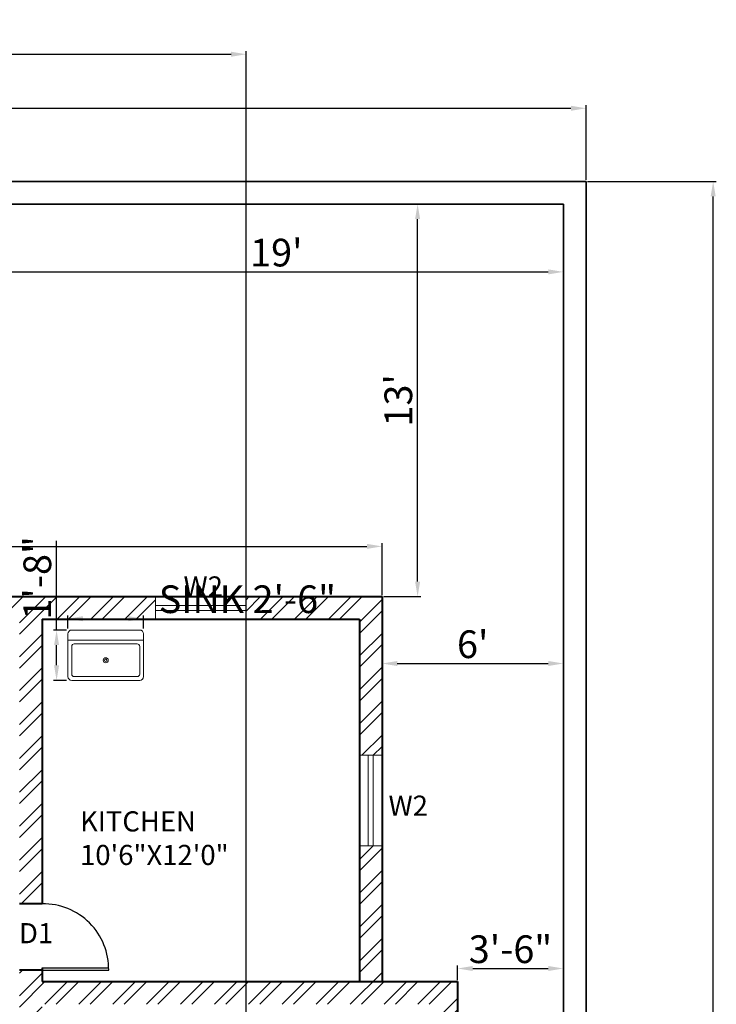
# Model space of a CAD drawing. Units: inches. Extents: x 2069 to 3028, y 691 to 1726.
# Tile 10 of 10: x 2622 to 2899, y 1325 to 1717. Entities that reach past the tile are written whole.
import ezdxf

# ---------------------------------------------------------------- set-up
doc = ezdxf.new("R2010")
doc.units = ezdxf.units.IN
for name, color, linetype, lineweight in [('A-ANNO-DIMS', 2, 'Continuous', 18), ('A-DOOR', 3, 'Continuous', 25), ('A-FLOR-FIXT', 9, 'Continuous', 20), ('A-GLAZ', 4, 'Continuous', 20), ('A-WALL', 7, 'Continuous', 40), ('L-SITE-WALL', 7, 'Continuous', 35)]:
    doc.layers.add(name, color=color, linetype=linetype, lineweight=lineweight)
for name, color, linetype, lineweight, true_color in [('A-ANNO-TEXT', 11, 'Continuous', 18, 0xf27172), ('A-AREA-IDEN', 11, 'Continuous', 25, 0xf27172), ('A-WALL-PATT', 143, 'Continuous', 13, 0x7aafdf)]:
    doc.layers.add(name, color=color, linetype=linetype, lineweight=lineweight, true_color=true_color)
doc.styles.get("Standard").update_dxf_attribs({"font": 'arial.ttf'})
doc.dimstyles.new('ISO-25', dxfattribs={"dimtxt": 11, "dimasz": 6, "dimexe": 1.25, "dimexo": 0.625, "dimtad": 1, "dimlunit": 3, "dimtxsty": 'Standard', "dimcen": 2.5, "dimclrd": 3, "dimclre": 5, "dimclrt": 6, "dimadec": 0, "dimazin": 0, "dimtfac": 1, "dimtmove": 0, "dimatfit": 3, "dimfxl": 1, "dimarcsym": 0})

# ---------------------------------------------------------------- blocks, each defined once
blk = doc.blocks.new('Sink-single - 30 in top')
blk.add_line((-15, -3.999996), (15, -3.999996))
for points in [[(-13.5, 0), (13.5, 0)], [(-15, -18.499996), (-15, -1.5)], [(15, -1.5), (15, -18.499996)], [(-13.5, -17.499996), (-13.5, -6.499996)], [(-12.5, -5.499996), (12.5, -5.499996)], [(13.5, -6.499996), (13.5, -17.499996)], [(12.5, -18.499996), (-12.5, -18.499996)], [(13.5, -19.999996), (-13.5, -19.999996)]]:
    blk.add_lwpolyline(points)
for radius in [1, 0.5]:
    blk.add_circle((0, -11.999996), radius)
for centre, radius, start, end in [((-13.5, -1.5), 1.5, 90, 180), ((13.5, -1.5), 1.5, 0, 90), ((-12.5, -6.499996), 1, 90, 180), ((12.5, -6.499996), 1, 0, 90), ((-13.5, -18.499996), 1.5, 180, 270), ((-12.5, -17.499996), 1, 180, 270), ((12.5, -17.499996), 1, 270, 0), ((13.5, -18.499996), 1.5, 270, 0)]:
    blk.add_arc(centre, radius, start, end)
blk = doc.blocks.new('*D20')
at = {"layer": 'A-ANNO-DIMS', "color": 0, "lineweight": -2, "transparency": 16777216}
for p, q in [((2141.95, 1653.01), (2141.95, 1682.68)), ((2846.95, 1653.01), (2846.95, 1682.68)), ((2147.95, 1681.43), (2840.95, 1681.43))]:
    blk.add_line(p, q, dxfattribs=at)
at = {"layer": 'A-ANNO-DIMS', "color": 0, "transparency": 16777216}
for points in [[(2147.95, 1682.43), (2147.95, 1680.43), (2141.95, 1681.43)], [(2840.95, 1682.43), (2840.95, 1680.43), (2846.95, 1681.43)]]:
    blk.add_solid(points, dxfattribs=at)
at = {"layer": 'Defpoints', "color": 0, "transparency": 16777216}
for p in [(2846.95, 1681.43), (2141.95, 1652.39), (2846.95, 1652.39)]:
    blk.add_point(p, dxfattribs=at)
at = {"layer": 'A-ANNO-DIMS', "color": 0, "transparency": 16777216, "insert": (2494.45, 1687.67), "char_height": 11, "attachment_point": 5}
blk.add_mtext('58\'-9"', dxfattribs=at)
blk = doc.blocks.new('*D21')
at = {"layer": 'A-ANNO-DIMS', "color": 0, "lineweight": -2, "transparency": 16777216}
for p, q in [((2766.58, 1643.39), (2781.31, 1643.39)), ((2780.06, 1493.39), (2780.06, 1637.39)), ((2766.58, 1487.39), (2781.31, 1487.39))]:
    blk.add_line(p, q, dxfattribs=at)
at = {"layer": 'A-ANNO-DIMS', "color": 0, "transparency": 16777216}
for points in [[(2779.06, 1637.39), (2781.06, 1637.39), (2780.06, 1643.39)], [(2779.06, 1493.39), (2781.06, 1493.39), (2780.06, 1487.39)]]:
    blk.add_solid(points, dxfattribs=at)
at = {"layer": 'Defpoints', "color": 0, "transparency": 16777216}
for p in [(2765.95, 1643.39), (2780.06, 1643.39), (2765.95, 1487.39)]:
    blk.add_point(p, dxfattribs=at)
at = {"layer": 'A-ANNO-DIMS', "color": 0, "transparency": 16777216, "insert": (2773.82, 1565.39), "char_height": 11, "attachment_point": 5, "rotation": 90}
blk.add_mtext("13'", dxfattribs=at)
blk = doc.blocks.new('*D22')
at = {"layer": 'A-ANNO-DIMS', "color": 0, "lineweight": -2, "transparency": 16777216}
for p, q in [((2609.95, 1642.76), (2609.95, 1615.16)), ((2837.95, 1642.76), (2837.95, 1615.16)), ((2615.95, 1616.41), (2831.95, 1616.41))]:
    blk.add_line(p, q, dxfattribs=at)
at = {"layer": 'A-ANNO-DIMS', "color": 0, "transparency": 16777216}
for points in [[(2615.95, 1617.41), (2615.95, 1615.41), (2609.95, 1616.41)], [(2831.95, 1617.41), (2831.95, 1615.41), (2837.95, 1616.41)]]:
    blk.add_solid(points, dxfattribs=at)
at = {"layer": 'Defpoints', "color": 0, "transparency": 16777216}
for p in [(2609.95, 1643.39), (2837.95, 1643.39), (2837.95, 1616.41)]:
    blk.add_point(p, dxfattribs=at)
at = {"layer": 'A-ANNO-DIMS', "color": 0, "transparency": 16777216, "insert": (2723.95, 1622.65), "char_height": 11, "attachment_point": 5}
blk.add_mtext("19'", dxfattribs=at)
blk = doc.blocks.new('*D23')
at = {"layer": 'A-ANNO-DIMS', "color": 0, "lineweight": -2, "transparency": 16777216}
for p, q in [((2297.95, 1488.01), (2297.95, 1508.59)), ((2303.95, 1507.34), (2759.95, 1507.34)), ((2765.95, 1488.01), (2765.95, 1508.59))]:
    blk.add_line(p, q, dxfattribs=at)
at = {"layer": 'A-ANNO-DIMS', "color": 0, "transparency": 16777216}
for points in [[(2303.95, 1508.34), (2303.95, 1506.34), (2297.95, 1507.34)], [(2759.95, 1508.34), (2759.95, 1506.34), (2765.95, 1507.34)]]:
    blk.add_solid(points, dxfattribs=at)
at = {"layer": 'Defpoints', "color": 0, "transparency": 16777216}
for p in [(2765.95, 1507.34), (2297.95, 1487.39), (2765.95, 1487.39)]:
    blk.add_point(p, dxfattribs=at)
at = {"layer": 'A-ANNO-DIMS', "color": 0, "transparency": 16777216, "insert": (2531.95, 1513.58), "char_height": 11, "attachment_point": 5}
blk.add_mtext("39'", dxfattribs=at)
blk = doc.blocks.new('*D24')
at = {"layer": 'A-ANNO-DIMS', "color": 0, "lineweight": -2, "transparency": 16777216}
for p, q in [((2795.95, 1335.01), (2795.95, 1340.86)), ((2801.95, 1339.61), (2831.95, 1339.61)), ((2837.95, 1335.01), (2837.95, 1340.86))]:
    blk.add_line(p, q, dxfattribs=at)
at = {"layer": 'A-ANNO-DIMS', "color": 0, "transparency": 16777216}
for points in [[(2801.95, 1340.61), (2801.95, 1338.61), (2795.95, 1339.61)], [(2831.95, 1340.61), (2831.95, 1338.61), (2837.95, 1339.61)]]:
    blk.add_solid(points, dxfattribs=at)
at = {"layer": 'Defpoints', "color": 0, "transparency": 16777216}
for p in [(2837.95, 1339.61), (2795.95, 1334.39), (2837.95, 1334.39)]:
    blk.add_point(p, dxfattribs=at)
at = {"layer": 'A-ANNO-DIMS', "color": 0, "transparency": 16777216, "insert": (2816.95, 1345.85), "char_height": 11, "attachment_point": 5}
blk.add_mtext('3\'-6"', dxfattribs=at)
blk = doc.blocks.new('*D25')
at = {"layer": 'A-ANNO-DIMS', "color": 0, "lineweight": -2, "transparency": 16777216}
for p, q in [((2765.95, 1486.76), (2765.95, 1459.55)), ((2837.95, 1486.76), (2837.95, 1459.55)), ((2771.95, 1460.8), (2831.95, 1460.8))]:
    blk.add_line(p, q, dxfattribs=at)
at = {"layer": 'A-ANNO-DIMS', "color": 0, "transparency": 16777216}
for points in [[(2771.95, 1461.8), (2771.95, 1459.8), (2765.95, 1460.8)], [(2831.95, 1461.8), (2831.95, 1459.8), (2837.95, 1460.8)]]:
    blk.add_solid(points, dxfattribs=at)
at = {"layer": 'Defpoints', "color": 0, "transparency": 16777216}
for p in [(2765.95, 1487.39), (2837.95, 1487.39), (2837.95, 1460.8)]:
    blk.add_point(p, dxfattribs=at)
at = {"layer": 'A-ANNO-DIMS', "color": 0, "transparency": 16777216, "insert": (2801.95, 1467.04), "char_height": 11, "attachment_point": 5}
blk.add_mtext("6'", dxfattribs=at)
blk = doc.blocks.new('DOOR-SWING-26_4IN')
for p, q in [((0, 0), (-26.4, 0)), ((0, -1), (-26.4, -1))]:
    blk.add_line(p, q)
blk.add_arc((-0.5, -0.5), 25.9, 178.894, 271.106)
blk = doc.blocks.new('WINDOW-36IN')
for p, q in [((0, 0), (9, 0)), ((3.5, 0), (3.5, -36)), ((5.5, 0), (5.5, -36)), ((0, -36), (9, -36))]:
    blk.add_line(p, q)
blk = doc.blocks.new('*D74')
at = {"layer": 'A-ANNO-DIMS', "color": 5, "lineweight": -2, "transparency": 16777216}
for p, q in [((2641.15, 1474.73), (2641.15, 1479.86)), ((2671.15, 1474.73), (2671.15, 1479.86))]:
    blk.add_line(p, q, dxfattribs=at)
at = {"layer": 'A-ANNO-DIMS', "color": 3, "lineweight": -2, "transparency": 16777216}
for p, q in [((2647.15, 1478.61), (2665.15, 1478.61)), ((2671.15, 1478.61), (2747.73, 1478.61))]:
    blk.add_line(p, q, dxfattribs=at)
at = {"layer": 'A-ANNO-DIMS', "color": 3, "transparency": 16777216}
for points in [[(2647.15, 1479.61), (2647.15, 1477.61), (2641.15, 1478.61)], [(2665.15, 1479.61), (2665.15, 1477.61), (2671.15, 1478.61)]]:
    blk.add_solid(points, dxfattribs=at)
at = {"layer": 'Defpoints', "color": 0, "transparency": 16777216}
for p in [(2671.15, 1478.61), (2641.15, 1474.11), (2671.15, 1474.11)]:
    blk.add_point(p, dxfattribs=at)
at = {"layer": 'A-ANNO-DIMS', "color": 6, "transparency": 16777216, "insert": (2712.44, 1484.92), "char_height": 11, "attachment_point": 5}
blk.add_mtext('SINK 2\'-6"', dxfattribs=at)
blk = doc.blocks.new('*D75')
at = {"layer": 'A-ANNO-DIMS', "color": 3, "lineweight": -2, "transparency": 16777216}
for p, q in [((2636.65, 1474.11), (2636.65, 1509.56)), ((2636.65, 1460.11), (2636.65, 1468.11))]:
    blk.add_line(p, q, dxfattribs=at)
at = {"layer": 'A-ANNO-DIMS', "color": 5, "lineweight": -2, "transparency": 16777216}
for p, q in [((2640.53, 1474.11), (2635.4, 1474.11)), ((2640.53, 1454.11), (2635.4, 1454.11))]:
    blk.add_line(p, q, dxfattribs=at)
at = {"layer": 'A-ANNO-DIMS', "color": 3, "transparency": 16777216}
for points in [[(2635.65, 1468.11), (2637.65, 1468.11), (2636.65, 1474.11)], [(2635.65, 1460.11), (2637.65, 1460.11), (2636.65, 1454.11)]]:
    blk.add_solid(points, dxfattribs=at)
at = {"layer": 'Defpoints', "color": 0, "transparency": 16777216}
for p in [(2636.65, 1474.11), (2641.15, 1474.11), (2641.15, 1454.11)]:
    blk.add_point(p, dxfattribs=at)
at = {"layer": 'A-ANNO-DIMS', "color": 6, "transparency": 16777216, "insert": (2630.41, 1494.84), "char_height": 11, "attachment_point": 5, "rotation": 90}
blk.add_mtext('1\'-8"', dxfattribs=at)
blk = doc.blocks.new('*D86')
at = {"layer": 'A-ANNO-DIMS', "color": 5, "lineweight": -2, "transparency": 16777216}
for p, q in [((2847.58, 1652.39), (2898.7, 1652.39)), ((2847.58, 737.39), (2898.7, 737.39))]:
    blk.add_line(p, q, dxfattribs=at)
at = {"layer": 'A-ANNO-DIMS', "color": 3, "lineweight": -2, "transparency": 16777216}
blk.add_line((2897.45, 743.39), (2897.45, 1646.39), dxfattribs=at)
at = {"layer": 'A-ANNO-DIMS', "color": 3, "transparency": 16777216}
for points in [[(2896.45, 1646.39), (2898.45, 1646.39), (2897.45, 1652.39)], [(2896.45, 743.39), (2898.45, 743.39), (2897.45, 737.39)]]:
    blk.add_solid(points, dxfattribs=at)
at = {"layer": 'Defpoints', "color": 0, "transparency": 16777216}
for p in [(2846.95, 1652.39), (2897.45, 1652.39), (2846.95, 737.39)]:
    blk.add_point(p, dxfattribs=at)
at = {"layer": 'A-ANNO-DIMS', "color": 6, "transparency": 16777216, "insert": (2891.21, 1194.89), "char_height": 11, "attachment_point": 5, "rotation": 90}
blk.add_mtext('76\'-3"', dxfattribs=at)
blk = doc.blocks.new('*D89')
at = {"layer": 'A-ANNO-DIMS', "color": 5, "lineweight": -2, "transparency": 16777216}
for p, q in [((2336.92, 747.01), (2336.92, 1704.14)), ((2711.95, 747.01), (2711.95, 1704.14))]:
    blk.add_line(p, q, dxfattribs=at)
at = {"layer": 'A-ANNO-DIMS', "color": 3, "lineweight": -2, "transparency": 16777216}
blk.add_line((2342.92, 1702.89), (2705.95, 1702.89), dxfattribs=at)
at = {"layer": 'A-ANNO-DIMS', "color": 3, "transparency": 16777216}
for points in [[(2342.92, 1703.89), (2342.92, 1701.89), (2336.92, 1702.89)], [(2705.95, 1703.89), (2705.95, 1701.89), (2711.95, 1702.89)]]:
    blk.add_solid(points, dxfattribs=at)
at = {"layer": 'Defpoints', "color": 0, "transparency": 16777216}
for p in [(2711.95, 1702.89), (2336.92, 746.39), (2711.95, 746.39)]:
    blk.add_point(p, dxfattribs=at)
at = {"layer": 'A-ANNO-DIMS', "color": 6, "transparency": 16777216, "insert": (2524.44, 1709.13), "char_height": 11, "attachment_point": 5}
blk.add_mtext('31\'-3"', dxfattribs=at)

msp = doc.modelspace()

# ---------------------------------------------------------------- hatches: boundary and pattern name
at = {"layer": 'A-WALL-PATT'}
h = msp.add_hatch(dxfattribs=at)
h.set_pattern_fill('ANSI32', color=256)
h.paths.add_polyline_path([(2675.951, 1487.387), (2576.951, 1487.387), (2576.951, 1478.387), (2621.951, 1478.387), (2621.951, 1365.287), (2630.951, 1365.287), (2630.951, 1478.387), (2675.951, 1478.387)])
h.paths.add_polyline_path([(2765.951, 1487.387), (2711.951, 1487.387), (2711.951, 1478.387), (2756.951, 1478.387), (2756.951, 1424.387), (2765.951, 1424.387)])
h.paths.add_polyline_path([(2528.951, 1487.387), (2407.751, 1487.387), (2407.751, 1478.387), (2474.951, 1478.387), (2474.951, 1434.887), (2498.951, 1434.887), (2498.951, 1374.887), (2474.951, 1374.887), (2474.951, 1365.287), (2483.951, 1365.287), (2483.951, 1370.387), (2507.951, 1370.387), (2507.951, 1439.387), (2483.951, 1439.387), (2483.951, 1478.387), (2528.951, 1478.387)])
h.paths.add_polyline_path([(2374.151, 1487.387), (2297.951, 1487.387), (2297.951, 1424.387), (2306.951, 1424.387), (2306.951, 1478.387), (2374.151, 1478.387)])
h.paths.add_polyline_path([(2507.951, 1334.387), (2483.951, 1334.387), (2483.951, 1338.887), (2474.951, 1338.887), (2474.951, 1334.387), (2306.951, 1334.387), (2306.951, 1388.387), (2297.951, 1388.387), (2297.951, 1334.387), (2267.951, 1334.387), (2267.951, 1274.387), (2276.951, 1274.387), (2276.951, 1325.387), (2297.951, 1325.387), (2423.951, 1325.387), (2423.951, 1187.387), (2419.451, 1187.387), (2419.451, 1178.387), (2432.951, 1178.387), (2432.951, 1325.387), (2507.951, 1325.387)])
h.paths.add_polyline_path([(2795.951, 1334.387), (2630.951, 1334.387), (2630.951, 1338.887), (2621.951, 1338.887), (2621.951, 1178.387), (2635.451, 1178.387), (2635.451, 1187.387), (2630.951, 1187.387), (2630.951, 1325.387), (2786.951, 1325.387), (2786.951, 1274.387), (2795.951, 1274.387)])
h.paths.add_polyline_path([(2765.951, 1388.387), (2756.951, 1388.387), (2756.951, 1334.387), (2765.951, 1334.387)])
h.paths.add_polyline_path([(2795.951, 1238.387), (2786.951, 1238.387), (2786.951, 1187.387), (2665.451, 1187.387), (2665.451, 1178.387), (2795.951, 1178.387)], flags=17)
h.paths.add_polyline_path([(2389.451, 1187.387), (2276.951, 1187.387), (2276.951, 1238.387), (2267.951, 1238.387), (2267.951, 1178.387), (2297.951, 1178.387), (2297.951, 1173.287), (2307.451, 1173.287), (2307.451, 1178.387), (2389.451, 1178.387)])
h.paths.add_polyline_path([(2377.451, 1142.387), (2306.951, 1142.387), (2306.951, 1146.887), (2297.951, 1146.887), (2297.951, 1142.387), (2297.951, 1137.887), (2306.951, 1137.887), (2372.951, 1137.887), (2372.951, 1133.387), (2377.451, 1133.387)])
h.paths.add_polyline_path([(2795.951, 1065.887), (2665.451, 1065.887), (2665.451, 1056.887), (2786.951, 1056.887), (2786.951, 1002.887), (2795.951, 1002.887), (2795.951, 1056.887)])
h.paths.add_polyline_path([(2795.951, 966.887), (2786.951, 966.887), (2786.951, 912.887), (2732.951, 912.887), (2732.951, 903.887), (2795.951, 903.887)])
h.paths.add_polyline_path([(2483.951, 917.387), (2474.951, 917.387), (2474.951, 912.887), (2414.951, 912.887), (2414.951, 903.887), (2483.951, 903.887)])
h.paths.add_polyline_path([(2366.951, 912.887), (2306.951, 912.887), (2306.951, 960.887), (2297.951, 960.887), (2297.951, 903.887), (2366.951, 903.887)])
h.paths.add_polyline_path([(2498.951, 1056.887), (2498.951, 1065.887), (2377.451, 1065.887), (2377.451, 1111.787), (2372.951, 1111.787), (2372.951, 1065.887), (2306.951, 1065.887), (2306.951, 1116.287), (2297.951, 1116.287), (2297.951, 1056.887), (2297.951, 1008.887), (2306.951, 1008.887), (2306.951, 1056.887), (2474.951, 1056.887), (2474.951, 947.387), (2483.951, 947.387), (2483.951, 1056.887)])

# ---------------------------------------------------------------- linework, layer by layer
at = {"layer": 'A-WALL'}
for p, q in [((2297.951, 1487.387), (2765.951, 1487.387)), ((2765.951, 1487.387), (2765.951, 1334.387)), ((2630.951, 1478.387), (2630.951, 1365.287)), ((2630.951, 1478.387), (2756.951, 1478.387)), ((2756.951, 1478.387), (2756.951, 1334.387)), ((2630.951, 1365.287), (2621.951, 1365.287)), ((2630.951, 1338.887), (2621.951, 1338.887)), ((2630.951, 1339.887), (2630.951, 1334.387)), ((2630.951, 1334.387), (2795.951, 1334.387)), ((2795.951, 1334.387), (2795.951, 1178.387))]:
    msp.add_line(p, q, dxfattribs=at)
at = {"layer": 'L-SITE-WALL'}
for p, q in [((2141.951, 1652.387), (2846.951, 1652.387)), ((2846.951, 1652.387), (2846.951, 737.387)), ((2609.951, 1643.387), (2837.951, 1643.387)), ((2837.951, 1643.387), (2837.951, 1178.387)), ((2837.951, 1535.387), (2837.951, 1487.387))]:
    msp.add_line(p, q, dxfattribs=at)

# ---------------------------------------------------------------- block references
at = {"layer": 'A-DOOR', "rotation": 180}
msp.add_blockref('DOOR-SWING-26_4IN', (2630.951, 1338.887), dxfattribs=at)
at = {"layer": 'A-FLOR-FIXT'}
msp.add_blockref('Sink-single - 30 in top', (2656.154, 1474.108), dxfattribs=at)
at = {"layer": 'A-GLAZ'}
for p, rotation in [((2675.951, 1478.387), 89.99999999999812), ((2765.951, 1388.387), 180)]:
    msp.add_blockref('WINDOW-36IN', p, dxfattribs=dict(at, rotation=rotation))

# ---------------------------------------------------------------- texts
at = {"layer": 'A-ANNO-TEXT', "char_height": 8, "attachment_point": 1}
for s, insert in [('{\\fArial|b1|i0|c0|p34;W2}', (2687.078, 1495.419)), ('{\\fArial|b1|i0|c0|p34;W2}', (2768.511, 1408.313)), ('{\\fArial|b1|i0|c0|p34;D1}', (2621.727, 1357.651))]:
    msp.add_mtext_dynamic_manual_height_columns(s, width=34.05605, gutter_width=12.5, heights=[0], dxfattribs=dict(at, insert=insert))
at = {"layer": 'A-AREA-IDEN', "insert": (2645.983, 1402.071), "char_height": 8, "attachment_point": 1}
msp.add_mtext_dynamic_manual_height_columns('KITCHEN\\P10\'6"X12\'0"', width=119.20948, gutter_width=12.5, heights=[0], dxfattribs=at)

# ---------------------------------------------------------------- dimensions: what is measured, and where the dimension line sits
at = {"layer": 'A-ANNO-DIMS'}
for base, p1, p2, override, picture, middle in [((2711.951, 1702.887), (2336.919, 746.387), (2711.951, 746.387), {"dimdec": 1, "dimlfac": 1, "dimrnd": 0, "dimzin": 1, "dimdsep": 46, "dimlunit": 4, "dimfrac": 2}, '*D89', (2524.435, 1709.132)), ((2846.951, 1681.427), (2141.951, 1652.387), (2846.951, 1652.387), {"dimclrd": 0, "dimclre": 0, "dimclrt": 0}, '*D20', (2494.451, 1687.669)), ((2837.951, 1616.413), (2609.951, 1643.387), (2837.951, 1643.387), {"dimclrd": 0, "dimclre": 0, "dimclrt": 0}, '*D22', (2723.951, 1622.654)), ((2765.951, 1507.335), (2297.951, 1487.387), (2765.951, 1487.387), {"dimclrd": 0, "dimclre": 0, "dimclrt": 0}, '*D23', (2531.951, 1513.58)), ((2837.951, 1460.802), (2765.951, 1487.387), (2837.951, 1487.387), {"dimclrd": 0, "dimclre": 0, "dimclrt": 0}, '*D25', (2801.951, 1467.043)), ((2837.951, 1339.608), (2795.951, 1334.387), (2837.951, 1334.387), {"dimclrd": 0, "dimclre": 0, "dimclrt": 0}, '*D24', (2816.951, 1345.853))]:
    dim = msp.add_linear_dim(base=base, p1=p1, p2=p2, dimstyle='ISO-25', override=override, dxfattribs=at)
    dim.commit()
    dim.dimension.update_dxf_attribs({"geometry": picture, "text_midpoint": middle})
for base, p1, p2, override, picture, middle in [((2897.451, 1652.387), (2846.951, 737.387), (2846.951, 1652.387), {"dimdec": 1, "dimlfac": 1, "dimrnd": 0, "dimzin": 1, "dimdsep": 46, "dimlunit": 4, "dimfrac": 2}, '*D86', (2891.206, 1194.887)), ((2780.062, 1643.387), (2765.951, 1487.387), (2765.951, 1643.387), {"dimclrd": 0, "dimclre": 0, "dimclrt": 0}, '*D21', (2773.817, 1565.387)), ((2636.654, 1474.108), (2641.154, 1454.108), (2641.154, 1474.108), {"dimdec": 1, "dimlfac": 1, "dimrnd": 0, "dimzin": 1, "dimdsep": 46, "dimlunit": 4, "dimfrac": 2}, '*D75', (2630.413, 1494.836))]:
    dim = msp.add_linear_dim(base=base, p1=p1, p2=p2, angle=90, dimstyle='ISO-25', override=override, dxfattribs=at)
    dim.commit()
    dim.dimension.update_dxf_attribs({"geometry": picture, "text_midpoint": middle})
dim = msp.add_linear_dim(base=(2671.154, 1478.608), p1=(2641.154, 1474.108), p2=(2671.154, 1474.108), text='SINK <>', dimstyle='ISO-25', override={"dimdec": 1, "dimlfac": 1, "dimrnd": 0, "dimzin": 1, "dimdsep": 46, "dimlunit": 4, "dimfrac": 2}, dxfattribs=at)
dim.commit()
dim.dimension.update_dxf_attribs({"geometry": '*D74', "text_midpoint": (2712.441, 1484.921)})

doc.saveas('drawing.dxf')
